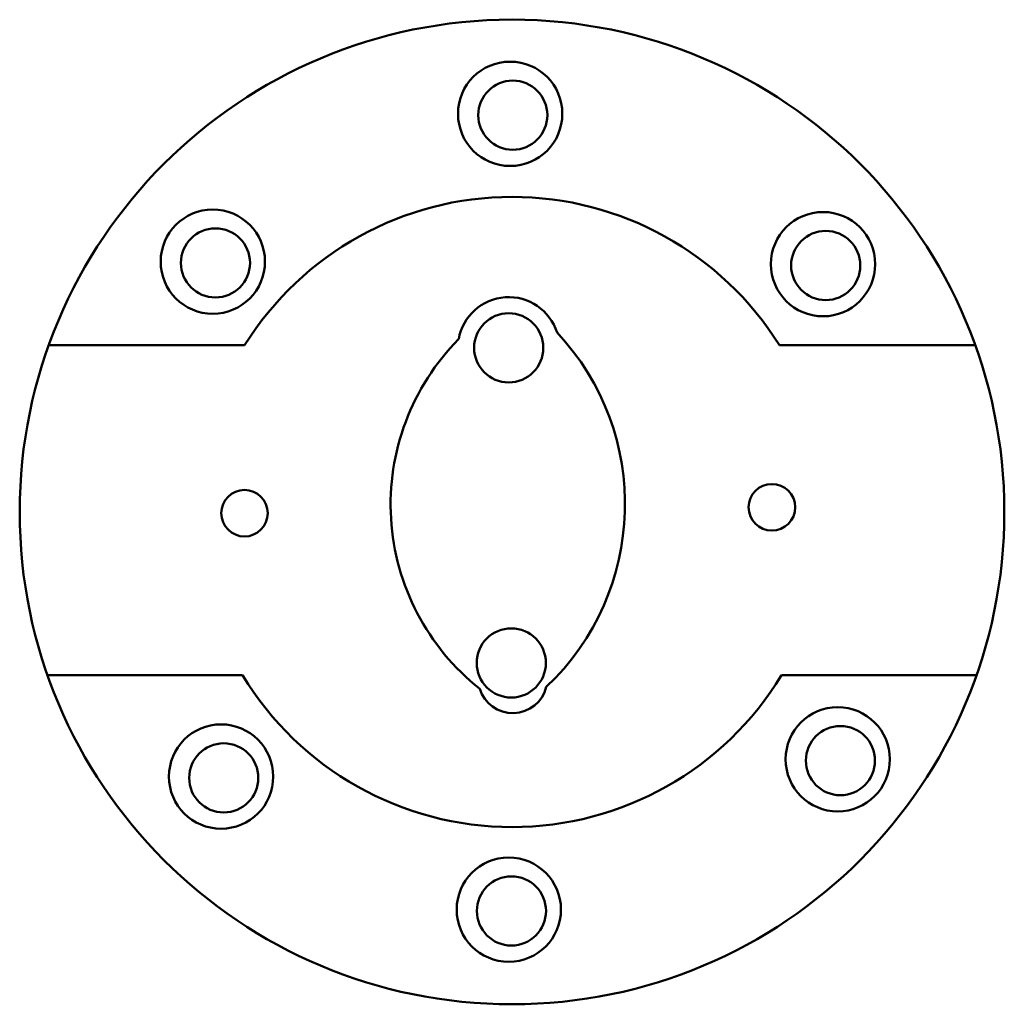
# Model space of a CAD drawing. Units: millimetres. Extents: x 2115 to 3650, y 1031 to 2567.
import ezdxf

# ---------------------------------------------------------------- set-up
doc = ezdxf.new("R2010")
doc.units = ezdxf.units.MM
doc.layers.add('M-OUTL', color=7, linetype='Continuous', lineweight=50)

# ---------------------------------------------------------------- blocks, each defined once
blk = doc.blocks.new('HOLE-CBORE')
for centre, radius in [((81.3, 81.3), 81.3), ((85.4, 79.2), 53.9)]:
    blk.add_circle(centre, radius)

msp = doc.modelspace()

# ---------------------------------------------------------------- linework, layer by layer
at = {"layer": 'M-OUTL'}
for p, q in [((2316.7, 2059), (2160.4, 2059)), ((2316.7, 2059), (2465.8, 2059)), ((3299.6, 2059), (3448.6, 2059)), ((3448.6, 2059), (3604.9, 2059)), ((2314.3, 1544.3), (2158.6, 1544.3)), ((2314.3, 1544.3), (2462.5, 1544.3)), ((3302.8, 1544.3), (3451, 1544.3)), ((3451, 1544.3), (3606.8, 1544.3))]:
    msp.add_line(p, q, dxfattribs=at)
for centre, radius in [((2882.7, 1799), 767.6), ((2877.5, 2054.9), 53.9), ((2877.5, 2054.9), 53.9), ((3287.9, 1806.3), 36.3), ((2465.6, 1797.1), 36.3), ((2881.6, 1563.6), 53.9)]:
    msp.add_circle(centre, radius, dxfattribs=at)
for centre, radius, start, end in [((2882.7, 1799), 491.3, 31.949, 148.051), ((2877.5, 2054.9), 79.1, 17.6295, 170.1369), ((2667.1, 1810.9), 391.7, 313.3778, 43.157), ((3059.7, 1810.6), 366.3, 135.2666, 231.6284), ((2882.7, 1799), 491.3, 211.2226, 328.7774), ((2883.9, 1539.3), 53.9, 197.0787, 345.879)]:
    msp.add_arc(centre, radius, start, end, dxfattribs=at)

# ---------------------------------------------------------------- block references
for p in [(2798.5, 2338.5), (2334.9, 2108.1), (3286.4, 2104.1), (3309.3, 1332.1), (2347.8, 1305.2), (2796.4, 1097.7)]:
    msp.add_blockref('HOLE-CBORE', p, dxfattribs=at)

doc.saveas('drawing.dxf')
